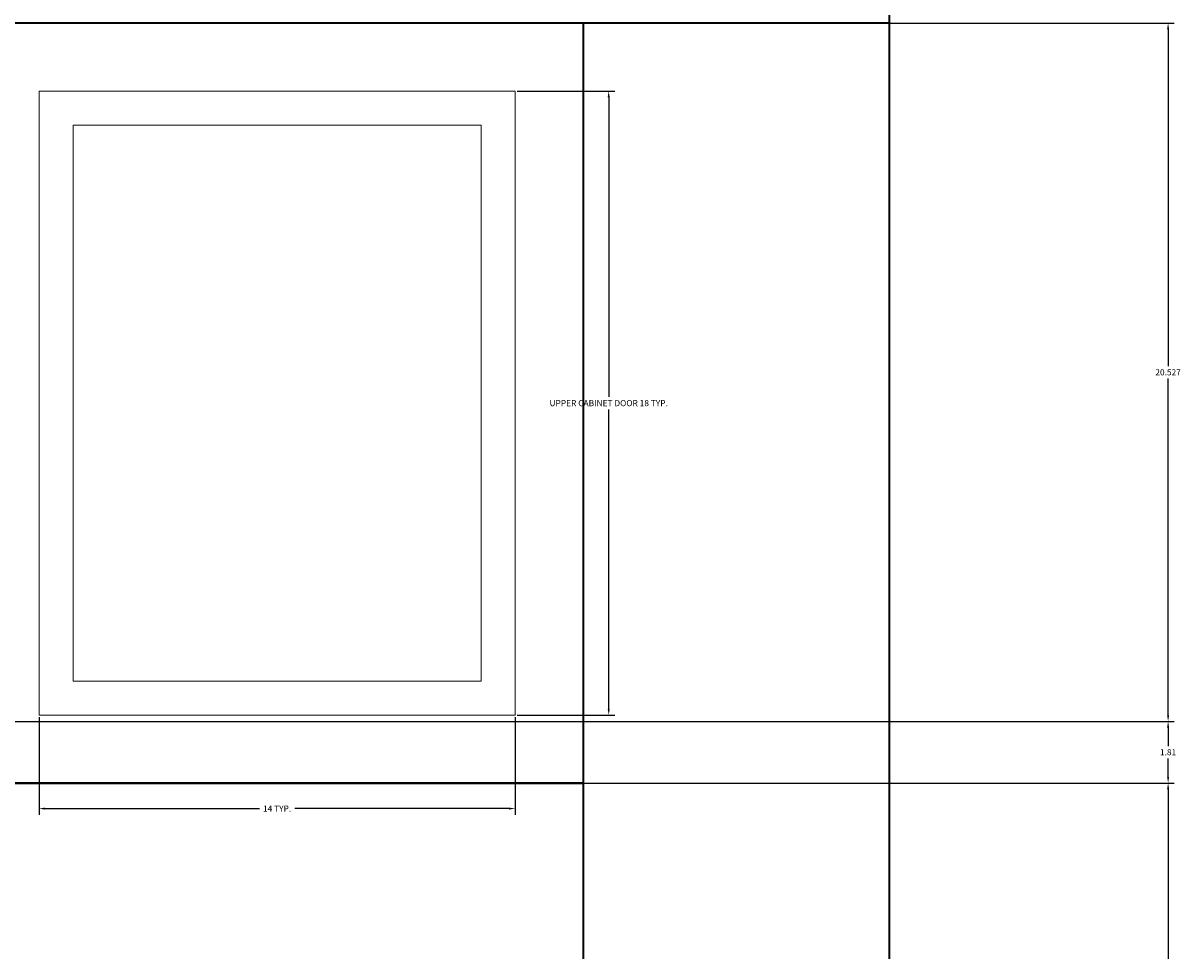
# Model space of a CAD drawing. Units: inches. Extents: x 27 to 200, y -50 to 102.
# Tile 25 of 26: x 166 to 200, y 61 to 88. Entities that reach past the tile are written whole.
import ezdxf

# ---------------------------------------------------------------- set-up
doc = ezdxf.new("R2010")
doc.units = ezdxf.units.IN
doc.header["$MEASUREMENT"] = 0
for name, color, linetype, lineweight in [('A-ANNO-DIMS', 2, 'Continuous', 18), ('A-ELEV', 7, 'Continuous', 35), ('A-FURN', 8, 'Continuous', 18)]:
    doc.layers.add(name, color=color, linetype=linetype, lineweight=lineweight)
doc.styles.get("Standard").update_dxf_attribs({"font": 'arial.ttf'})
doc.dimstyles.get("Standard").update_dxf_attribs({"dimtxt": 0.18, "dimasz": 0.18, "dimexe": 0.18, "dimexo": 0.0625, "dimgap": 0.09, "dimtad": 0, "dimtih": 1, "dimtoh": 1, "dimdec": 4, "dimzin": 0, "dimdsep": 46, "dimtxsty": 'Standard', "dimcen": 0.09, "dimadec": 0, "dimazin": 0, "dimtfac": 1, "dimtdec": 4, "dimtofl": 0, "dimtmove": 0, "dimatfit": 3, "dimfxl": 1, "dimtolj": 1, "dimtzin": 0, "dimarcsym": 0})

# ---------------------------------------------------------------- blocks, each defined once
blk = doc.blocks.new('CAB-DOOR-UPPER')
for p, q in [((0, 0), (0, 18.339)), ((0, 18.339), (14, 18.339)), ((14, 18.339), (14, 0)), ((1, 1), (1, 17.339)), ((1, 17.339), (13, 17.339)), ((13, 17.339), (13, 1)), ((13, 1), (1, 1)), ((14, 0), (0, 0))]:
    blk.add_line(p, q)
blk = doc.blocks.new('*D5')
at = {"layer": 'A-ANNO-DIMS', "color": 0, "lineweight": -2, "transparency": 16777216}
for p, q in [((180.479, 85.926), (183.348, 85.926)), ((183.168, 85.746), (183.168, 76.94)), ((183.168, 67.767), (183.168, 76.573)), ((180.479, 67.587), (183.348, 67.587))]:
    blk.add_line(p, q, dxfattribs=at)
at = {"layer": 'A-ANNO-DIMS', "color": 0, "transparency": 16777216}
for points in [[(183.138, 85.746), (183.198, 85.746), (183.168, 85.926)], [(183.138, 67.767), (183.198, 67.767), (183.168, 67.587)]]:
    blk.add_solid(points, dxfattribs=at)
at = {"layer": 'Defpoints', "color": 0, "transparency": 16777216}
for p in [(180.417, 85.926), (183.168, 85.926), (180.417, 67.587)]:
    blk.add_point(p, dxfattribs=at)
at = {"layer": 'A-ANNO-DIMS', "color": 0, "transparency": 16777216, "insert": (183.168, 76.756), "char_height": 0.18, "attachment_point": 5}
blk.add_mtext('\\A1;UPPER CABINET DOOR 18 TYP.', dxfattribs=at)
blk = doc.blocks.new('*D6')
at = {"layer": 'A-ANNO-DIMS', "color": 0, "lineweight": -2, "transparency": 16777216}
for p, q in [((166.417, 67.524), (166.417, 64.656)), ((180.417, 67.524), (180.417, 64.656)), ((166.597, 64.836), (172.897, 64.836)), ((180.237, 64.836), (173.937, 64.836))]:
    blk.add_line(p, q, dxfattribs=at)
at = {"layer": 'A-ANNO-DIMS', "color": 0, "transparency": 16777216}
for points in [[(166.597, 64.866), (166.597, 64.806), (166.417, 64.836)], [(180.237, 64.866), (180.237, 64.806), (180.417, 64.836)]]:
    blk.add_solid(points, dxfattribs=at)
at = {"layer": 'Defpoints', "color": 0, "transparency": 16777216}
for p in [(166.417, 67.587), (180.417, 67.587), (180.417, 64.836)]:
    blk.add_point(p, dxfattribs=at)
at = {"layer": 'A-ANNO-DIMS', "color": 0, "transparency": 16777216, "insert": (173.417, 64.836), "char_height": 0.18, "attachment_point": 5}
blk.add_mtext('\\A1;14 TYP.', dxfattribs=at)
blk = doc.blocks.new('*D29')
at = {"layer": 'A-ANNO-DIMS', "color": 0, "lineweight": -2, "transparency": 16777216}
for p, q in [((146.479, 65.587), (199.797, 65.587)), ((199.617, 65.407), (199.617, 58.938)), ((199.617, 52.106), (199.617, 58.575)), ((146.479, 51.926), (199.797, 51.926))]:
    blk.add_line(p, q, dxfattribs=at)
at = {"layer": 'A-ANNO-DIMS', "color": 0, "transparency": 16777216}
for points in [[(199.587, 65.407), (199.647, 65.407), (199.617, 65.587)], [(199.587, 52.106), (199.647, 52.106), (199.617, 51.926)]]:
    blk.add_solid(points, dxfattribs=at)
at = {"layer": 'Defpoints', "color": 0, "transparency": 16777216}
for p in [(146.417, 65.587), (199.617, 65.587), (146.417, 51.926)]:
    blk.add_point(p, dxfattribs=at)
at = {"layer": 'A-ANNO-DIMS', "color": 0, "transparency": 16777216, "insert": (199.617, 58.756), "char_height": 0.18, "attachment_point": 5}
blk.add_mtext('\\A1;13.66', dxfattribs=at)
blk = doc.blocks.new('*D30')
at = {"layer": 'A-ANNO-DIMS', "color": 0, "lineweight": -2, "transparency": 16777216}
for p, q in [((146.479, 67.399), (199.797, 67.399)), ((199.617, 67.219), (199.617, 66.675)), ((199.617, 65.767), (199.617, 66.311)), ((146.479, 65.587), (199.797, 65.587))]:
    blk.add_line(p, q, dxfattribs=at)
at = {"layer": 'A-ANNO-DIMS', "color": 0, "transparency": 16777216}
for points in [[(199.587, 67.219), (199.647, 67.219), (199.617, 67.399)], [(199.587, 65.767), (199.647, 65.767), (199.617, 65.587)]]:
    blk.add_solid(points, dxfattribs=at)
at = {"layer": 'Defpoints', "color": 0, "transparency": 16777216}
for p in [(146.417, 67.399), (199.617, 67.399), (146.417, 65.587)]:
    blk.add_point(p, dxfattribs=at)
at = {"layer": 'A-ANNO-DIMS', "color": 0, "transparency": 16777216, "insert": (199.617, 66.493), "char_height": 0.18, "attachment_point": 5}
blk.add_mtext('\\A1;1.81', dxfattribs=at)
blk = doc.blocks.new('*D31')
at = {"layer": 'A-ANNO-DIMS', "color": 0, "lineweight": -2, "transparency": 16777216}
for p, q in [((146.479, 87.926), (199.797, 87.926)), ((199.617, 87.746), (199.617, 77.845)), ((199.617, 67.579), (199.617, 77.481)), ((146.479, 67.399), (199.797, 67.399))]:
    blk.add_line(p, q, dxfattribs=at)
at = {"layer": 'A-ANNO-DIMS', "color": 0, "transparency": 16777216}
for points in [[(199.587, 87.746), (199.647, 87.746), (199.617, 87.926)], [(199.587, 67.579), (199.647, 67.579), (199.617, 67.399)]]:
    blk.add_solid(points, dxfattribs=at)
at = {"layer": 'Defpoints', "color": 0, "transparency": 16777216}
for p in [(146.417, 87.926), (199.617, 87.926), (146.417, 67.399)]:
    blk.add_point(p, dxfattribs=at)
at = {"layer": 'A-ANNO-DIMS', "color": 0, "transparency": 16777216, "insert": (199.617, 77.663), "char_height": 0.18, "attachment_point": 5}
blk.add_mtext('\\A1;20.527', dxfattribs=at)

msp = doc.modelspace()

# ---------------------------------------------------------------- linework, layer by layer
at = {"layer": 'A-ELEV'}
for p, q in [((191.4169, 93.9264), (191.4169, -16.7693)), ((191.4169, 87.9264), (35.4169, 87.9264)), ((182.4169, 87.9264), (182.4169, 65.5865)), ((182.4169, 65.5865), (146.4169, 65.5865)), ((146.4169, 65.5865), (182.4169, 65.5865)), ((164.4169, 65.5865), (182.4169, 65.5865)), ((182.4169, 65.5865), (182.4169, 19.0222))]:
    msp.add_line(p, q, dxfattribs=at)

# ---------------------------------------------------------------- block references
at = {"layer": 'A-FURN'}
msp.add_blockref('CAB-DOOR-UPPER', (166.417, 67.587), dxfattribs=at)

# ---------------------------------------------------------------- dimensions: what is measured, and where the dimension line sits
at = {"layer": 'A-ANNO-DIMS'}
for base, p1, p2, override, picture, middle in [((199.6169, 87.9264), (146.4169, 67.3991), (146.4169, 87.9264), {"dimdec": 3, "dimlfac": 1, "dimrnd": 0, "dimzin": 0, "dimdsep": 46, "dimlunit": 2}, '*D31', (199.6169, 77.6628)), ((199.6169, 67.3991), (146.4169, 65.5865), (146.4169, 67.3991), {"dimdec": 2, "dimlfac": 1, "dimrnd": 0, "dimzin": 0, "dimdsep": 46, "dimlunit": 2}, '*D30', (199.6169, 66.4928)), ((199.6169, 65.5865), (146.4169, 51.9264), (146.4169, 65.5865), {"dimdec": 2, "dimlfac": 1, "dimrnd": 0, "dimzin": 0, "dimdsep": 46, "dimlunit": 2}, '*D29', (199.6169, 58.7565))]:
    dim = msp.add_linear_dim(base=base, p1=p1, p2=p2, angle=90, dimstyle='Standard', override=override, dxfattribs=at)
    dim.commit()
    dim.dimension.update_dxf_attribs({"geometry": picture, "text_midpoint": middle})
dim = msp.add_linear_dim(base=(183.1679, 85.9264), p1=(180.4169, 67.5865), p2=(180.4169, 85.9264), angle=90, text='UPPER CABINET DOOR <> TYP.', dimstyle='Standard', override={"dimdec": 0, "dimrnd": 0, "dimzin": 0, "dimlunit": 2}, dxfattribs=at)
dim.commit()
dim.dimension.update_dxf_attribs({"geometry": '*D5', "text_midpoint": (183.1679, 76.7565)})
dim = msp.add_linear_dim(base=(180.4169, 64.8355), p1=(166.4169, 67.5865), p2=(180.4169, 67.5865), text='<> TYP.', dimstyle='Standard', override={"dimdec": 0, "dimrnd": 0, "dimzin": 0, "dimlunit": 2}, dxfattribs=at)
dim.commit()
dim.dimension.update_dxf_attribs({"geometry": '*D6', "text_midpoint": (173.4169, 64.8355)})

doc.saveas('drawing.dxf')
